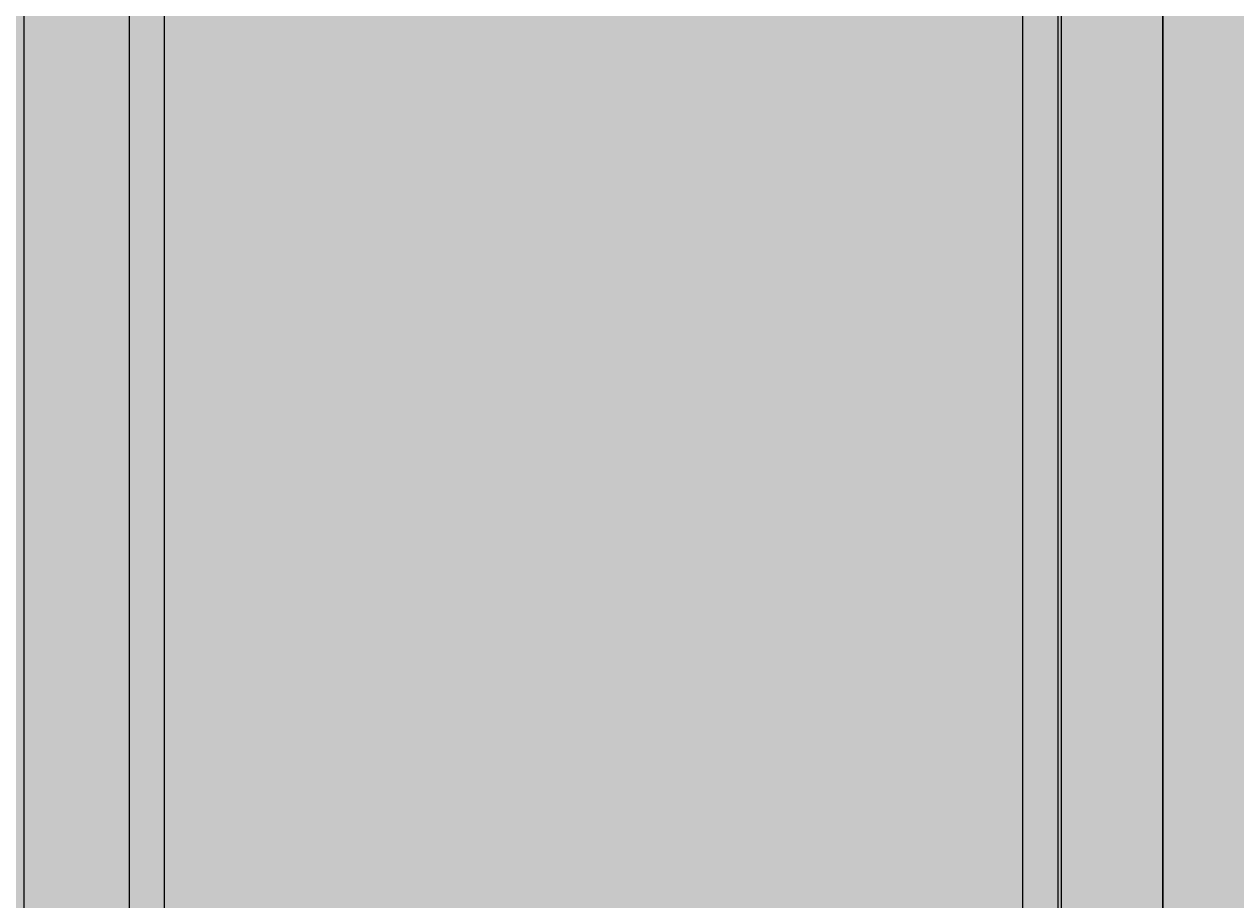
# Model space of a CAD drawing. Units: feet. Extents: x 2695 to 2912, y 795 to 1139.
# Tile 17 of 83: x 2774 to 2808, y 820 to 845. Entities that reach past the tile are written whole.
import ezdxf

# ---------------------------------------------------------------- set-up
doc = ezdxf.new("R2010")
doc.units = ezdxf.units.FT
for name, color, linetype, lineweight in [('A-ANNO-DIMS', 2, 'Continuous', 18), ('A-DOOR', 3, 'Continuous', 25), ('A-DOOR-PATT', 33, 'Continuous', 13), ('A-ELEV-PATT', 252, 'Continuous', 13)]:
    doc.layers.add(name, color=color, linetype=linetype, lineweight=lineweight)
doc.styles.get("Standard").update_dxf_attribs({"font": 'arial.ttf'})
doc.dimstyles.get("Standard").update_dxf_attribs({"dimtxt": 0.18, "dimasz": 0.18, "dimexe": 0.18, "dimexo": 0.0625, "dimgap": 0.09, "dimtad": 0, "dimtih": 1, "dimtoh": 1, "dimdec": 1, "dimzin": 0, "dimdsep": 46, "dimlunit": 3, "dimtxsty": 'Standard', "dimcen": 0.09, "dimadec": 0, "dimazin": 0, "dimtfac": 1, "dimtdec": 1, "dimtofl": 0, "dimtmove": 0, "dimatfit": 3, "dimfxl": 1, "dimtolj": 1, "dimtzin": 0, "dimarcsym": 0})

# ---------------------------------------------------------------- blocks, each defined once
blk = doc.blocks.new('*D13')
at = {"layer": 'A-ANNO-DIMS', "color": 0, "lineweight": -2, "transparency": 16777216}
for p, q in [((2758.214, 874.857), (2911.424, 874.857)), ((2911.244, 874.677), (2911.244, 843.076)), ((2911.244, 811.111), (2911.244, 842.712)), ((2890.699, 810.931), (2911.424, 810.931))]:
    blk.add_line(p, q, dxfattribs=at)
at = {"layer": 'A-ANNO-DIMS', "color": 0, "transparency": 16777216}
for points in [[(2911.214, 874.677), (2911.274, 874.677), (2911.244, 874.857)], [(2911.214, 811.111), (2911.274, 811.111), (2911.244, 810.931)]]:
    blk.add_solid(points, dxfattribs=at)
at = {"layer": 'Defpoints', "color": 0, "transparency": 16777216}
for p in [(2758.151, 874.857), (2911.244, 874.857), (2890.636, 810.931)]:
    blk.add_point(p, dxfattribs=at)
at = {"layer": 'A-ANNO-DIMS', "color": 0, "transparency": 16777216, "insert": (2911.244, 842.894), "char_height": 0.18, "attachment_point": 5}
blk.add_mtext('\\A1;63.93', dxfattribs=at)

msp = doc.modelspace()

# ---------------------------------------------------------------- hatches: boundary and pattern name
at = {"layer": 'A-DOOR-PATT'}
h = msp.add_hatch(color=256, dxfattribs=at)
h.set_gradient(color1=(211, 185, 150), color2=(211, 185, 150))
h.paths.add_polyline_path([(2805.9398, 905.5143), (2773.5029, 905.5143), (2773.5029, 810.9306), (2776.4999, 810.9306), (2776.4999, 902.5174), (2802.9429, 902.5174), (2802.9429, 810.9306), (2805.9398, 810.9306)])
h.paths.add_polyline_path([(2803.9681, 874.1057), (2805.0538, 874.1057), (2805.0538, 846.2857), (2803.9681, 846.2857)], flags=16)
h.paths.add_polyline_path([(2838.3767, 905.5143), (2805.9398, 905.5143), (2805.9398, 810.9306), (2808.9368, 810.9306), (2808.9368, 902.5174), (2835.3798, 902.5174), (2835.3798, 810.9306), (2838.3767, 810.9306)])
h = msp.add_hatch(color=256, dxfattribs=at)
h.set_gradient(color1=(211, 185, 150), color2=(211, 185, 150))
h.paths.add_polyline_path([(2777.5029, 901.5143), (2801.9398, 901.5143), (2801.9398, 810.9306), (2802.9429, 810.9306), (2802.9429, 902.5174), (2776.4999, 902.5174), (2776.4999, 810.9306), (2777.5029, 810.9306)])
h.paths.add_polyline_path([(2809.9398, 901.5143), (2834.3767, 901.5143), (2834.3767, 810.9306), (2835.3798, 810.9306), (2835.3798, 902.5174), (2808.9368, 902.5174), (2808.9368, 810.9306), (2809.9398, 810.9306)])
h = msp.add_hatch(color=256, dxfattribs=at)
h.set_gradient(color1=(173, 221, 247), color2=(173, 221, 247))
h.paths.add_polyline_path([(2801.9398, 901.5143), (2777.5029, 901.5143), (2777.5029, 810.9306), (2801.9398, 810.9306)])
h.paths.add_polyline_path([(2834.3767, 901.5143), (2809.9398, 901.5143), (2809.9398, 810.9306), (2834.3767, 810.9306)])
at = {"layer": 'A-ELEV-PATT'}
h = msp.add_hatch(color=256, dxfattribs=at)
h.set_gradient(color1=(147, 149, 152), color2=(147, 149, 152), tint=1)
h.paths.add_polyline_path([(2770.6361, 1118.4096), (2710.6361, 1118.4096), (2710.6361, 1062.9306), (2770.6361, 1062.9306)])
h.paths.add_polyline_path([(2890.6361, 1103.3378), (2770.6361, 1103.3378), (2770.6361, 1062.9306), (2890.6361, 1062.9306)])
h.paths.add_polyline_path([(2730.7081, 1048.1052), (2755.1125, 1048.1052), (2755.1125, 936.9306), (2770.6361, 936.9306), (2770.6361, 1050.3105), (2715.8852, 1050.3105), (2715.8852, 936.9306), (2730.7081, 936.9306)])
h.paths.add_polyline_path([(2890.6361, 1050.3105), (2770.6361, 1050.3105), (2770.6361, 971.9673), (2778.0341, 971.9673), (2778.0341, 1020.8235), (2843.575, 1020.8235), (2843.575, 971.9673), (2890.6361, 971.9673)])
h.paths.add_polyline_path([(2888.1882, 970.7156), (2843.575, 970.7156), (2843.575, 964.8267), (2888.1882, 964.8267)])
h.paths.add_polyline_path([(2888.1882, 964.1328), (2843.575, 964.1328), (2843.575, 956.614), (2888.1882, 956.614)])
h.paths.add_polyline_path([(2888.1882, 955.9202), (2843.575, 955.9202), (2843.575, 949.2892), (2888.1882, 949.2892)])
h.paths.add_polyline_path([(2888.1882, 948.5954), (2843.575, 948.5954), (2843.575, 941.3507), (2888.1882, 941.3507)])
h.paths.add_polyline_path([(2888.1882, 940.6569), (2843.575, 940.6569), (2843.575, 936.9306), (2888.1882, 936.9306)])
h.paths.add_polyline_path([(2890.6361, 970.7156), (2888.9368, 970.7156), (2888.9368, 964.8267), (2890.6361, 964.8267)])
h.paths.add_polyline_path([(2890.6361, 964.1328), (2888.9368, 964.1328), (2888.9368, 956.614), (2890.6361, 956.614)])
h.paths.add_polyline_path([(2890.6361, 955.9202), (2888.9368, 955.9202), (2888.9368, 949.2892), (2890.6361, 949.2892)])
h.paths.add_polyline_path([(2890.6361, 940.6569), (2888.9368, 940.6569), (2888.9368, 936.9306), (2890.6361, 936.9306)])
h.paths.add_polyline_path([(2890.6361, 948.5954), (2888.9368, 948.5954), (2888.9368, 941.3507), (2890.6361, 941.3507)])
h.paths.add_polyline_path([(2772.5216, 970.7156), (2770.6361, 970.7156), (2770.6361, 964.8267), (2772.5216, 964.8267)])
h.paths.add_polyline_path([(2772.5216, 964.1328), (2770.6361, 964.1328), (2770.6361, 956.614), (2772.5216, 956.614)])
h.paths.add_polyline_path([(2772.5216, 955.9202), (2770.6361, 955.9202), (2770.6361, 949.2892), (2772.5216, 949.2892)])
h.paths.add_polyline_path([(2772.5216, 948.5954), (2770.6361, 948.5954), (2770.6361, 941.3507), (2772.5216, 941.3507)])
h.paths.add_polyline_path([(2772.5216, 940.6569), (2770.6361, 940.6569), (2770.6361, 936.9306), (2772.5216, 936.9306)])
h.paths.add_polyline_path([(2778.0341, 940.6569), (2773.2702, 940.6569), (2773.2702, 936.9306), (2778.0341, 936.9306)])
h.paths.add_polyline_path([(2778.0341, 970.7156), (2773.2702, 970.7156), (2773.2702, 964.8267), (2778.0341, 964.8267)])
h.paths.add_polyline_path([(2778.0341, 964.1328), (2773.2702, 964.1328), (2773.2702, 956.614), (2778.0341, 956.614)])
h.paths.add_polyline_path([(2778.0341, 955.9202), (2773.2702, 955.9202), (2773.2702, 949.2892), (2778.0341, 949.2892)])
h.paths.add_polyline_path([(2778.0341, 948.5954), (2773.2702, 948.5954), (2773.2702, 941.3507), (2778.0341, 941.3507)])
h.paths.add_polyline_path([(2810.0407, 940.6569), (2780.0341, 940.6569), (2780.0341, 936.9306), (2810.0407, 936.9306)])
h.paths.add_polyline_path([(2890.6361, 924.3105), (2770.6361, 924.3105), (2770.6361, 810.9306), (2773.5029, 810.9306), (2773.5029, 905.5143), (2805.9398, 905.5143), (2838.3767, 905.5143), (2838.3767, 810.9306), (2890.6361, 810.9306)])

# ---------------------------------------------------------------- linework, layer by layer
at = {"layer": 'A-DOOR'}
for points in [[(2773.5029, 810.9306), (2773.5029, 905.5143), (2805.9398, 905.5143), (2805.9398, 810.9306)], [(2838.3767, 810.9306), (2838.3767, 905.5143), (2805.9398, 905.5143), (2805.9398, 810.9306)], [(2776.4999, 810.9306), (2776.4999, 902.5174), (2802.9429, 902.5174), (2802.9429, 810.9306)], [(2777.5029, 810.9306), (2777.5029, 901.5143), (2801.9398, 901.5143), (2801.9398, 810.9306)]]:
    msp.add_lwpolyline(points, dxfattribs=at)
for points in [[(2773.5029, 905.5143), (2838.3767, 905.5143), (2838.3767, 810.9306), (2773.5029, 810.9306)], [(2805.9398, 905.5143), (2805.9398, 905.5143), (2805.9398, 810.9306), (2805.9398, 810.9306)], [(2776.4999, 902.5174), (2803.0393, 902.5174), (2803.0393, 810.9306), (2776.4999, 810.9306)], [(2777.5029, 901.5143), (2801.9398, 901.5143), (2801.9398, 810.9306), (2777.5029, 810.9306)]]:
    msp.add_lwpolyline(points, close=True, dxfattribs=at)

# ---------------------------------------------------------------- dimensions: what is measured, and where the dimension line sits
at = {"layer": 'A-ANNO-DIMS'}
dim = msp.add_linear_dim(base=(2911.2444, 874.8571), p1=(2890.6361, 810.9306), p2=(2758.1515, 874.8571), angle=90, dimstyle='Standard', override={"dimdec": 2, "dimlfac": 1, "dimrnd": 0, "dimzin": 0, "dimdsep": 46, "dimlunit": 2}, dxfattribs=at)
dim.commit()
dim.dimension.update_dxf_attribs({"geometry": '*D13', "text_midpoint": (2911.2444, 842.8938)})

doc.saveas('drawing.dxf')
